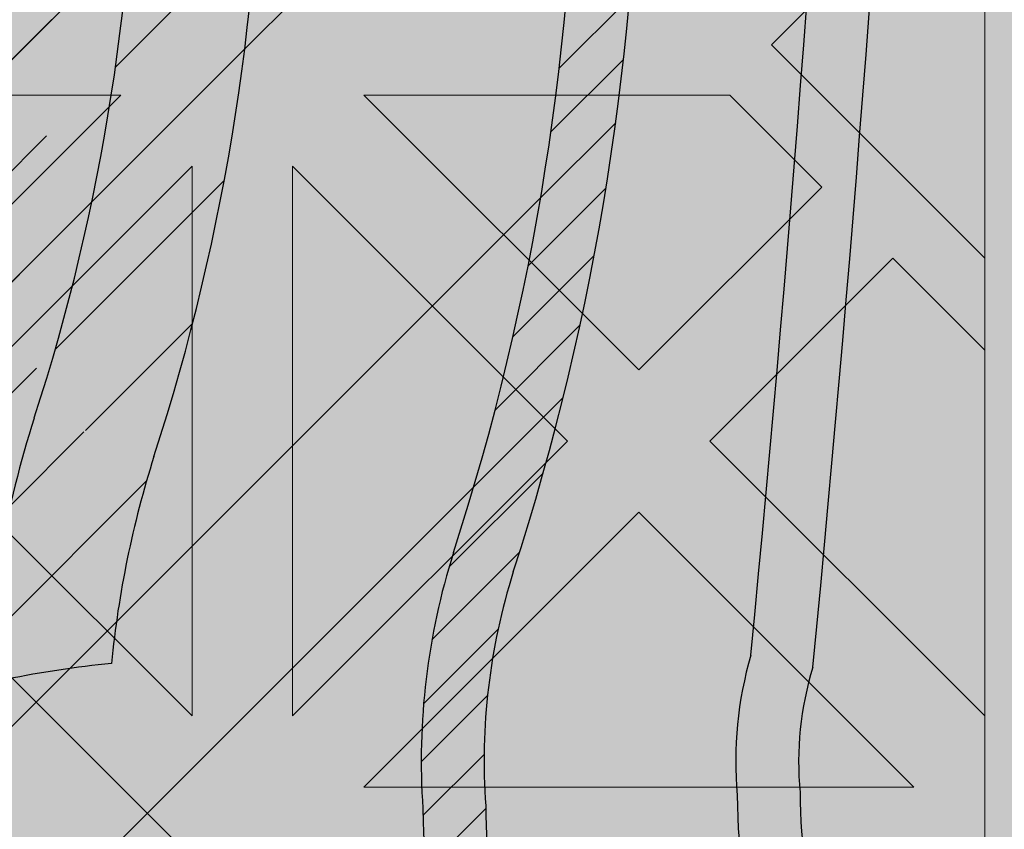
# Model space of a CAD drawing. Units: inches. Extents: x 844 to 2234, y 346 to 1084.
# Tile 54 of 93: x 1871.357 to 1873.853, y 694.275 to 696.327. Entities that reach past the tile are written whole.
import ezdxf

# ---------------------------------------------------------------- set-up
doc = ezdxf.new("R2010")
doc.units = ezdxf.units.IN
doc.header["$MEASUREMENT"] = 0
doc.layers.add('furniture', color=8, linetype='Continuous', lineweight=18)
doc.layers.add('RA-AP-01$0$INT', color=35, linetype='Continuous', lineweight=5)
doc.layers.add('RA-AP-01$0$FURN', color=3, linetype='Continuous')
doc.layers.add('RA-AP-01$0$WOOD', color=64, linetype='Continuous')

# ---------------------------------------------------------------- blocks, each defined once
blk = doc.blocks.new('A$C18D01794')
at = {"layer": 'RA-AP-01$0$INT'}
blk.add_hatch(color=256, dxfattribs=at).paths.add_polyline_path([(4.505206456958071, -6.306712009588038), (5.305206456958072, -6.306712009588038), (5.305206456958072, -7.106712009588038), (5.255206456951893, -7.10671200958804), (5.25520645694868, -6.356712009605972), (4.555206456959269, -6.356712009587461), (4.555206456956052, -7.106712009588038), (4.505206456958073, -7.106712009588038)])
h = blk.add_hatch(color=256, dxfattribs=at)
h.paths.add_polyline_path([(4.585917135068449, -6.356712009588271), (4.555206456959269, -6.35671200958746), (4.555206456959137, -6.387422687716308), (4.874495778835233, -6.706712009592356), (4.90520645695423, -6.676001331474049)])
h.paths.add_polyline_path([(5.255206456948813, -6.387422687716306), (5.255206456948682, -6.356712009605972), (5.224495778822613, -6.356712009605161), (4.905206456953498, -6.676001331474273), (4.935917135072151, -6.706712009592924)])
h.paths.add_polyline_path([(4.935917135072559, -6.706712009592068), (4.905206456953564, -6.737422687710376), (5.255206456951813, -7.087422687708613), (5.255206456951549, -7.026001331471008)])
h.paths.add_polyline_path([(4.555206456956399, -7.026001331471013), (4.555206456956134, -7.087422687708616), (4.905206456953821, -6.737422687710943), (4.874495778835166, -6.70671200959229)])
h = blk.add_hatch(color=256, dxfattribs=at)
h.paths.add_polyline_path([(4.585917135068448, -6.356712009588273), (4.614201406330596, -6.356712009589021), (4.668846067270487, -6.411356670531338), (4.723490728212344, -6.356712009591912), (4.771774999457151, -6.35671200959319), (4.826419660396886, -6.411356670535356), (4.862780050090322, -6.374996280843536), (4.844495778842715, -6.356712009595112), (4.862780050090411, -6.356712009595595), (4.905206456960182, -6.399138416468211), (4.947632863832445, -6.356712009597838), (4.965917135079675, -6.356712009598322), (4.947632863831759, -6.374996280845421), (4.983993253523576, -6.411356670538857), (5.038637914464627, -6.356712009600247), (5.08692218571208, -6.356712009601523), (5.141566846649976, -6.411356670541852), (5.196211507589851, -6.356712009604411), (5.224495778822615, -6.356712009605161), (4.905206456953975, -6.676001331473793)])
h.paths.add_polyline_path([(4.895206456956031, -6.637717060225675), (4.895206456958921, -6.528427738347902), (4.840561796018589, -6.583072399285802)], flags=16)
h.paths.add_polyline_path([(4.915206456955638, -6.637717060226121), (4.969851117895509, -6.583072399288678), (4.915206456957609, -6.528427738348344)], flags=16)
h.paths.add_polyline_path([(4.826419660395175, -6.568930263661755), (4.881064321335613, -6.514285602723745), (4.771774999456703, -6.514285602720857)], flags=16)
h.paths.add_polyline_path([(4.983993253519558, -6.568930263665262), (5.038637914460456, -6.514285602726792), (4.929348592581548, -6.514285602724816)], flags=16)
h.paths.add_polyline_path([(4.881064321336025, -6.494285602723742), (4.826419660397532, -6.439640941782821), (4.771774999457062, -6.494285602720859)], flags=16)
h.paths.add_polyline_path([(4.929348592582019, -6.494285602724817), (5.038637914460982, -6.494285602726792), (4.983993253522945, -6.439640941786327)], flags=16)
h.paths.add_polyline_path([(4.895206456960191, -6.480143467100443), (4.895206456962115, -6.407422687715913), (4.876922185715016, -6.389138416467584), (4.840561796021581, -6.425498806159401)], flags=16)
h.paths.add_polyline_path([(4.915206456958487, -6.480143467100889), (4.969851117899527, -6.425498806162279), (4.933490728206909, -6.389138416468043), (4.9152064569598, -6.40742268771434)], flags=16)
h.paths.add_polyline_path([(4.757632863832376, -6.480143467096812), (4.812277524772842, -6.425498806158772), (4.757632863834348, -6.370854145217844)], flags=16)
h.paths.add_polyline_path([(4.737632863832376, -6.480143467096286), (4.737632863834348, -6.370854145217375), (4.682988202893906, -6.425498806155385)], flags=16)
h.paths.add_polyline_path([(5.05278005008503, -6.480143467103376), (5.052780050087917, -6.370854145224413), (4.998135389146995, -6.425498806162908)], flags=16)
h.paths.add_polyline_path([(5.072780050085024, -6.480143467103744), (5.127424711025931, -6.42549880616527), (5.072780050087916, -6.370854145224832)], flags=16)
h.paths.add_polyline_path([(4.935917135072783, -6.706712009592292), (5.255206456948811, -6.387422687716309), (5.255206456948932, -6.415706958964177), (5.200561796010279, -6.470351619902839), (5.255206456949403, -6.524996280841948), (5.25520645694961, -6.5732805520894), (5.200561796009787, -6.627925213029239), (5.236922185702417, -6.664285602721864), (5.255206456949919, -6.646001331474357), (5.255206456949998, -6.664285602721898), (5.212780050078687, -6.706712009592262), (5.25520645695036, -6.749138416463932), (5.255206456950438, -6.767422687711313), (5.236922185702424, -6.749138416463297), (5.200561796009796, -6.785498806155928), (5.255206456950753, -6.840143467096874), (5.25520645695096, -6.888427738341682), (5.200561796010322, -6.943072399282328), (5.255206456951428, -6.997717060223427), (5.255206456951547, -7.026001331471006)])
h.paths.add_polyline_path([(5.042988202883395, -6.785498806155427), (5.097632863823085, -6.840143467095101), (5.097632863822622, -6.730854145216193)], flags=16)
h.paths.add_polyline_path([(5.028846067259663, -6.771356670531693), (5.083490728198774, -6.716712009592573), (4.974201406321001, -6.716712009593042)], flags=16)
h.paths.add_polyline_path([(5.117632863823087, -6.840143467095186), (5.172277524762331, -6.785498806155926), (5.11763286382262, -6.730854145216225)], flags=16)
h.paths.add_polyline_path([(5.08349072819877, -6.696712009593886), (5.028846067259652, -6.642067348654775), (4.974201406320998, -6.696712009593438)], flags=16)
h.paths.add_polyline_path([(5.131774999446817, -6.854285602718917), (5.186419660386065, -6.799640941779662), (5.241064321325782, -6.854285602719365)], flags=17)
h.paths.add_polyline_path([(5.131774999446228, -6.716712009592374), (5.186419660386065, -6.771356670532194), (5.222780050079488, -6.734996280838764), (5.204495778832781, -6.716712009592063)], flags=16)
h.paths.add_polyline_path([(5.097632863822613, -6.682569873970264), (5.097632863823061, -6.573280552091354), (5.042988202883383, -6.627925213031044)], flags=16)
h.paths.add_polyline_path([(5.131774999446899, -6.874285602718915), (5.241064321325809, -6.874285602719364), (5.186419660386591, -6.928930263658598)], flags=17)
h.paths.add_polyline_path([(5.131774999446226, -6.696712009594078), (5.204495778830767, -6.696712009594374), (5.22278005007868, -6.67842773834687), (5.186419660386049, -6.642067348654249)], flags=16)
h.paths.add_polyline_path([(5.11763286382262, -6.682569873970225), (5.17227752476232, -6.627925213030515), (5.117632863823064, -6.573280552091267)], flags=16)
h.paths.add_polyline_path([(5.186419660386069, -6.613783077405491), (5.241064321325754, -6.559138416465795), (5.131774999446791, -6.559138416466263)], flags=16)
h.paths.add_polyline_path([(5.131774999446872, -6.539138416466263), (5.24106432132578, -6.539138416465794), (5.186419660386554, -6.484493755526573)], flags=16)
h.paths.add_polyline_path([(5.255206456951811, -7.08742268770861), (5.255206456951895, -7.106712009588038), (4.555206456956052, -7.106712009588038), (4.555206456956136, -7.087422687708617), (4.905206456953973, -6.737422687710788)])
h.paths.add_polyline_path([(4.983993253513404, -6.8444937555241), (4.92934859257295, -6.899138416462108), (5.03863791445186, -6.899138416465014)], flags=16)
h.paths.add_polyline_path([(4.969851117889988, -6.83035161990006), (4.915206456952556, -6.775706958960171), (4.915206456949648, -6.884996280837944)], flags=16)
h.paths.add_polyline_path([(4.929348592572535, -6.919138416462105), (4.983993253511019, -6.973783077403037), (5.038637914451496, -6.919138416465012)], flags=16)
h.paths.add_polyline_path([(5.052780050074912, -6.93328055208906), (4.998135389134438, -6.987925213027088), (5.052780050072919, -7.042569873968025)], flags=16)
h.paths.add_polyline_path([(5.07278005007491, -6.933280552089588), (5.072780050072918, -7.042569873968497), (5.127424711013374, -6.987925213030498)], flags=16)
h.paths.add_polyline_path([(4.89520645695295, -6.775706958959721), (4.840561796013067, -6.830351619897157), (4.895206456950961, -6.884996280837494)], flags=16)
h.paths.add_polyline_path([(4.915206456948365, -6.933280552085403), (4.915206456946434, -7.006001331471951), (4.933490728192729, -7.024285602719066), (4.969851117886972, -6.987925213026453)], flags=16)
h.paths.add_polyline_path([(4.881064321327021, -6.899138416461022), (4.82641966038902, -6.84449375552057), (4.771774999448108, -6.899138416459029)], flags=16)
h.paths.add_polyline_path([(4.895206456950073, -6.933280552084951), (4.840561796009022, -6.987925213023558), (4.876922185700835, -7.024285602716997), (4.895206456948749, -7.006001331469487)], flags=16)
h.paths.add_polyline_path([(4.983993253510392, -7.0020673486505), (4.947632863816944, -7.038427738342319), (4.965917135064043, -7.05671200959023), (5.038637914448995, -7.056712009591555)], flags=16)
h.paths.add_polyline_path([(4.881064321326543, -6.91913841646102), (4.771774999447578, -6.919138416459031), (4.826419660385607, -6.973783077399508)], flags=16)
h.paths.add_polyline_path([(4.905206456946447, -7.014285602717636), (4.862780050074785, -7.056712009588352), (4.947632863816685, -7.056712009589775)], flags=16)
h.paths.add_polyline_path([(5.14156684663679, -7.002067348654549), (5.086922185696452, -7.056712009592438), (5.196211507574223, -7.056712009594425)], flags=16)
h.paths.add_polyline_path([(4.8264196603837, -7.002067348646972), (4.771774999442643, -7.056712009585575), (4.8444957788276, -7.056712009587508), (4.862780050075511, -7.038427738340416)], flags=16)
h.paths.add_polyline_path([(4.812277524760289, -6.98792521302292), (4.757632863822258, -6.933280552082447), (4.757632863819352, -7.042569873961408)], flags=16)
h.paths.add_polyline_path([(4.73763286382226, -6.933280552082079), (4.682988202881349, -6.987925213020536), (4.737632863819352, -7.04256987396099)], flags=16)
h.paths.add_polyline_path([(4.723490728195188, -7.056712009584289), (4.668846067257299, -7.002067348643949), (4.614201406317417, -7.056712009581383)], flags=16)
h.paths.add_polyline_path([(4.597632863829262, -6.706712009592262), (4.555206456957951, -6.664285602721896), (4.555206456958029, -6.646001331474357), (4.573490728205535, -6.664285602721864), (4.609851117898167, -6.627925213029238), (4.555206456958338, -6.573280552089402), (4.555206456958546, -6.524996280841952), (4.60985111789767, -6.470351619902839), (4.555206456959015, -6.415706958964177), (4.555206456959138, -6.387422687716309), (4.874495778835167, -6.70671200959229), (4.5552064569564, -7.026001331471015), (4.555206456956523, -6.997717060223433), (4.609851117897629, -6.94307239928233), (4.555206456956988, -6.888427738341681), (4.555206456957198, -6.840143467096881), (4.609851117898153, -6.78549880615593), (4.573490728205528, -6.749138416463297), (4.555206456957507, -6.76742268771132), (4.555206456957585, -6.749138416463933)])
h.paths.add_polyline_path([(4.712780050085332, -6.730854145216195), (4.712780050084863, -6.840143467095105), (4.767424711024555, -6.785498806155427)], flags=16)
h.paths.add_polyline_path([(4.726922185709173, -6.716712009592573), (4.781566846648288, -6.771356670531693), (4.836211507586949, -6.716712009593043)], flags=16)
h.paths.add_polyline_path([(4.692780050085327, -6.730854145216225), (4.638135389145619, -6.785498806155928), (4.692780050084865, -6.840143467095185)], flags=16)
h.paths.add_polyline_path([(4.726922185709182, -6.696712009593886), (4.836211507586949, -6.696712009593436), (4.7815668466483, -6.642067348654773)], flags=16)
h.paths.add_polyline_path([(4.678637914461726, -6.71671200959237), (4.605917135075169, -6.716712009592063), (4.587632863828464, -6.734996280838766), (4.623993253521887, -6.771356670532195)], flags=16)
h.paths.add_polyline_path([(4.712780050085336, -6.68256987397026), (4.767424711024568, -6.627925213031042), (4.71278005008489, -6.573280552091352)], flags=16)
h.paths.add_polyline_path([(4.678637914461726, -6.696712009594076), (4.623993253521899, -6.642067348654247), (4.587632863829271, -6.67842773834687), (4.605917135077185, -6.696712009594376)], flags=16)
h.paths.add_polyline_path([(4.692780050085336, -6.682569873970228), (4.692780050084889, -6.573280552091267), (4.638135389145632, -6.627925213030515)], flags=16)
h.paths.add_polyline_path([(4.623993253521885, -6.799640941779662), (4.678637914461131, -6.854285602718915), (4.56934859258217, -6.854285602719365)], flags=17)
h.paths.add_polyline_path([(4.623993253521901, -6.613783077405509), (4.678637914461158, -6.559138416466263), (4.569348592582195, -6.559138416465795)], flags=16)
h.paths.add_polyline_path([(4.678637914461051, -6.874285602718915), (4.623993253521361, -6.928930263658598), (4.569348592582143, -6.874285602719364)], flags=17)
h.paths.add_polyline_path([(4.678637914461076, -6.539138416466263), (4.623993253521399, -6.484493755526573), (4.569348592582167, -6.539138416465796)], flags=16)
h = blk.add_hatch(color=256, dxfattribs=at)
h.paths.add_polyline_path([(5.028846067259997, -6.642067348655121), (4.974201406321342, -6.696712009593783), (5.083490728199115, -6.69671200959423)])
h.paths.add_polyline_path([(4.974201406321344, -6.716712009593388), (5.028846067260004, -6.771356670532039), (5.083490728199117, -6.716712009592919)])
h.paths.add_polyline_path([(5.042988202883738, -6.785498806155768), (5.097632863823428, -6.840143467095449), (5.097632863822963, -6.73085414521654)])
h.paths.add_polyline_path([(5.117632863822961, -6.730854145216568), (5.117632863823428, -6.840143467095531), (5.172277524762674, -6.785498806156272)])
h.paths.add_polyline_path([(5.131774999446572, -6.716712009592718), (5.186419660386406, -6.77135667053254), (5.222780050079831, -6.734996280839116), (5.204495778833122, -6.716712009592409)])
h.paths.add_polyline_path([(5.236922185702764, -6.749138416463644), (5.200561796010139, -6.785498806156274), (5.255206456949971, -6.840143467096101), (5.255206456950271, -6.76742268771115)])
h.paths.add_polyline_path([(5.186419660386412, -6.799640941780006), (5.131774999447164, -6.854285602719262), (5.241064321326123, -6.854285602719711)])
h.paths.add_polyline_path([(5.131774999447238, -6.874285602719261), (5.186419660386934, -6.928930263658944), (5.241064321326153, -6.874285602719709)])
h.paths.add_polyline_path([(5.200561796010663, -6.943072399282675), (5.255206456949324, -6.997717060221329), (5.255206456949777, -6.888427738343558)])
h.paths.add_polyline_path([(5.21278005007903, -6.706712009592607), (5.255206456950223, -6.749138416463798), (5.255206456950696, -6.664285602721891)])
h.paths.add_polyline_path([(5.13177499944657, -6.696712009594424), (5.204495778831106, -6.696712009594723), (5.222780050079024, -6.678427738347219), (5.186419660386397, -6.642067348654592)])
h.paths.add_polyline_path([(5.117632863823405, -6.573280552091611), (5.117632863822955, -6.682569873970578), (5.172277524762665, -6.627925213030859)])
h.paths.add_polyline_path([(5.042988202883727, -6.627925213031387), (5.097632863822957, -6.682569873970603), (5.097632863823407, -6.573280552091697)])
h.paths.add_polyline_path([(5.131774999447135, -6.559138416466609), (5.186419660386394, -6.613783077405857), (5.241064321326097, -6.559138416466144)])
h.paths.add_polyline_path([(5.200561796010128, -6.627925213029584), (5.236922185702758, -6.664285602722211), (5.255206456950264, -6.646001331474705), (5.255206456949948, -6.573280552089752)])
h.paths.add_polyline_path([(5.186419660386895, -6.484493755526919), (5.131774999447213, -6.539138416466609), (5.241064321326127, -6.539138416466142)])
h.paths.add_polyline_path([(5.200561796010624, -6.470351619903183), (5.255206456949745, -6.524996280842298), (5.255206456949276, -6.415706958964523)])
for p, q in [((5.255206456951895, -7.106712009588038), (5.255206456948681, -6.356712009605972)), ((4.935917135072783, -6.706712009592292), (5.255206456948813, -6.387422687716307)), ((5.131774999446792, -6.559138416466263), (5.241064321325755, -6.559138416465795)), ((5.131774999446792, -6.559138416466263), (5.186419660386049, -6.613783077405509)), ((5.241064321325755, -6.559138416465795), (5.186419660386049, -6.613783077405509)), ((5.042988202883385, -6.627925213031041), (5.097632863823062, -6.573280552091352)), ((5.097632863823062, -6.573280552091352), (5.097632863822615, -6.682569873970262)), ((5.117632863823062, -6.573280552091267), (5.172277524762319, -6.627925213030515)), ((5.117632863823062, -6.573280552091267), (5.117632863822614, -6.68256987397023)), ((5.255206456949605, -6.573280552089405), (5.200561796009783, -6.627925213029239)), ((5.255206456949918, -6.646001331474357), (5.255206456949605, -6.573280552089405)), ((5.097632863822615, -6.682569873970262), (5.042988202883383, -6.627925213031042)), ((5.117632863822614, -6.68256987397023), (5.172277524762319, -6.627925213030515)), ((5.200561796009783, -6.627925213029238), (5.236922185702415, -6.664285602721863)), ((5.083490728198769, -6.696712009593882), (5.028846067259652, -6.642067348654775)), ((5.131774999446228, -6.696712009594078), (5.186419660386053, -6.642067348654247)), ((5.186419660386051, -6.642067348654247), (5.222780050078681, -6.67842773834687)), ((5.255206456949919, -6.646001331474357), (5.236922185702415, -6.664285602721864)), ((5.212780050078687, -6.706712009592262), (5.255206456950353, -6.664285602721543)), ((5.25520645694988, -6.74913841646345), (5.255206456950353, -6.664285602721543)), ((5.204495778833082, -6.69671200959206), (5.222780050078681, -6.67842773834687)), ((5.08349072819877, -6.696712009593886), (4.974201406320999, -6.696712009593436)), ((5.204495778831179, -6.696712009594376), (5.131774999446228, -6.696712009594078)), ((5.212780050078687, -6.706712009592262), (5.25520645694988, -6.74913841646345))]:
    blk.add_line(p, q, dxfattribs=at)
blk = doc.blocks.new('A$C32926AE1')
at = {"layer": 'RA-AP-01$0$FURN'}
h = blk.add_hatch(dxfattribs=at)
h.set_pattern_fill('ANSI31', color=256, scale=0.1, style=0)
h.set_pattern_definition([(45, (0, 0), (-0.0088388347648318, 0.0088388347648318), [])])
edge = h.paths.add_edge_path(flags=16)
edge.add_arc((4.904771284329206, 4.246793130718756), 0.2603971832811541, 75.22398030683196, 104.7760196931204)
edge.add_arc((4.904771284329206, 4.246793130718756), 0.2603971832811541, 75.223980306832, 104.77601969312039, ccw=False)
edge = h.paths.add_edge_path(flags=16)
edge.add_arc((4.904771284329206, 4.067062675376612), 0.2603971832811541, 255.2239803068796, 284.776019693168)
edge.add_arc((4.904771284329206, 4.067062675376612), 0.2603971832811541, 255.22398030687958, 284.77601969316805, ccw=False)
edge = h.paths.add_edge_path(flags=0)
edge.add_arc((4.904771284329206, 4.067062675376612), 0.2603971832811541, 255.2239803068796, 284.776019693168)
edge.add_arc((4.904771284329206, 4.067062675376612), 0.2603971832811541, 255.22398030687958, 284.77601969316805, ccw=False)
edge = h.paths.add_edge_path(flags=0)
edge.add_arc((4.904771284329206, 4.067062675376612), 0.2603971832811541, 255.2239803068796, 284.776019693168)
edge.add_arc((4.904771284329206, 4.067062675376612), 0.2603971832811541, 255.22398030687958, 284.77601969316805, ccw=False)
edge = h.paths.add_edge_path()
edge.add_arc((4.604388392048174, 4.588829985554312), 0.1599999999999918, 342.3781640246255, 354.4317409793762)
edge.add_arc((5.090145208887507, 4.43216705527679), 0.3503971832811637, 162.0091218307731, 180.3186872093483)
edge.add_arc((5.205154176610243, 4.588829985554953), 0.1599999999999917, 185.5682590208461, 197.6218359767349)
edge.add_arc((4.904771284329229, 4.246793130718735), 0.3503971832811761, 72.00912183053516, 107.9908781690354)
edge.add_arc((9.535952835716557, 4.28682295566602), 4.798342501046485, 178.2875002453811, 181.5576802719453)
edge.add_arc((4.719397359771122, 4.43216705527679), 0.3503971832811637, 359.6813127906516, 377.9908781692269)
edge.add_arc((9.535967292294904, 4.286822350292874), 4.778371420254705, 178.2965938931842, 181.5667745797229)
edge.add_arc((4.719397359771122, 4.43216705527679), 0.3303971832811637, 359.6813127906516, 377.9908781692269)
edge.add_arc((0.2735752763637294, 4.286822350292874), 4.7783714202547, 358.4332254202771, 361.7034061068158)
edge.add_arc((5.061434214606998, 4.732549947558029), 0.1600000000000254, 252.3781640250584, 264.4317409792362)
edge.add_arc((4.748108354051257, 4.732549947558012), 0.1600000000000541, 275.5682590208426, 287.6218359759532)
edge.add_arc((4.604388392048115, 4.588829985554317), 0.1800000000000505, 342.3567572500182, 349.3735009646207)
edge.add_arc((5.205154176610254, 4.588829985554976), 0.1800000000000069, 190.6264990356027, 197.6432427513933)
edge.add_arc((5.061434214607106, 4.732549947558013), 0.1800000000000424, 252.3567572496606, 259.3735009644582)
edge.add_arc((4.904771284329208, 4.246793130718737), 0.3303971832811676, 71.99844483668534, 108.0015551637021)
edge.add_arc((4.748108354051414, 4.732549947558045), 0.1800000000000547, 280.6264990355479, 287.6432427495938)
edge.add_arc((5.090145208887514, 4.432167055276789), 0.2803971832811691, 162.8706300666893, 180.816523289902)
edge.add_arc((4.719397359771136, 4.432167055276689), 0.2803971832811534, 359.183476710103, 377.1293699333214)
edge.add_arc((4.904771284329222, 4.246793130718737), 0.2803971832811769, 72.87063006672916, 107.1293699332334)
edge.add_arc((5.090145208887522, 4.432167055276788), 0.2603971832811776, 165.2239803068007, 180.9953123810312)
edge.add_arc((4.719397359771141, 4.432167055276699), 0.2603971832811458, 359.0046876189768, 374.7760196932087)
edge.add_arc((5.090145208887507, 4.43216705527679), 0.3303971832811637, 162.0091218307731, 180.3186872093483)
edge.add_arc((9.53595427642584, 4.285015535491528), 4.728345371032053, 178.265043920078, 181.5679956281801)
edge.add_arc((0.2735882922327999, 4.285015535491582), 4.728345371032045, 358.4320043718193, 361.7349560799204)
edge.add_arc((9.535953591267507, 4.284458026472751), 4.708343996644348, 178.2573054306777, 181.5704995759608)
edge.add_arc((0.273588977391114, 4.284458026472785), 4.708343996644358, 358.4295004240388, 361.7426945693213)
edge.add_arc((0.2735889773911131, 4.029397779622582), 4.708343996644359, 358.2573054306787, 361.5704995759613)
edge.add_arc((9.535953591267518, 4.029397779622618), 4.708343996644359, 178.4295004240391, 181.7426945693223)
edge.add_arc((0.2735882922327901, 4.028840270603786), 4.728345371032054, 358.2650439200796, 361.5679956281808)
edge.add_arc((9.53595427642584, 4.028840270603841), 4.728345371032054, 178.4320043718199, 181.7349560799219)
edge.add_arc((0.2735752763637302, 4.027033455802493), 4.778371420254699, 358.2965938931842, 361.5667745797229)
edge.add_arc((4.719397359771122, 3.881688750818578), 0.3303971832811637, 342.0091218307731, 360.3186872093484)
edge.add_arc((5.090145208887507, 3.881688750818578), 0.3303971832811637, 179.6813127906516, 197.9908781692269)
edge.add_arc((9.535967292294904, 4.027033455802493), 4.778371420254705, 178.433225420277, 181.7034061068158)
edge.add_arc((4.719397359771122, 3.881688750818578), 0.3503971832811637, 342.0091218307731, 360.3186872093484)
edge.add_arc((9.53595283571655, 4.027032850429349), 4.79834250104648, 178.4423197280546, 181.7124997546188)
edge.add_arc((4.719397359771141, 3.881688750818669), 0.2603971832811458, 345.2239803067913, 360.9953123810232)
edge.add_arc((5.090145208887522, 3.88168875081858), 0.2603971832811776, 179.0046876189687, 194.7760196931993)
edge.add_arc((4.904771284329222, 4.067062675376631), 0.2803971832811769, 252.8706300667665, 287.1293699332708)
edge.add_arc((4.719397359771136, 3.881688750818678), 0.2803971832811534, 342.8706300666787, 360.8165232898969)
edge.add_arc((5.090145208887514, 3.881688750818579), 0.2803971832811691, 179.183476710098, 197.1293699333106)
edge.add_arc((4.748108354051414, 3.581305858537323), 0.1800000000000547, 72.3567572504062, 79.37350096445199)
edge.add_arc((4.904771284329208, 4.067062675376631), 0.3303971832811676, 251.9984448362979, 288.0015551633146)
edge.add_arc((5.061434214607106, 3.581305858537355), 0.1800000000000424, 100.6264990355418, 107.6432427503394)
edge.add_arc((5.205154176610254, 3.725025820540392), 0.1800000000000069, 162.3567572486066, 169.3735009643972)
edge.add_arc((4.604388392048115, 3.725025820541051), 0.1800000000000505, 10.62649903537925, 17.64324274998182)
edge.add_arc((4.748108354051257, 3.581305858537356), 0.1600000000000541, 72.37816402404681, 84.43174097915735)
edge.add_arc((4.904771284329229, 4.067062675376632), 0.3503971832811761, 252.0091218309645, 287.9908781694648)
edge.add_arc((5.061434214606998, 3.581305858537339), 0.1600000000000254, 95.56825902076373, 107.6218359749416)
edge.add_arc((5.205154176610243, 3.725025820540414), 0.1599999999999917, 162.3781640232651, 174.4317409791539)
edge.add_arc((5.090145208887507, 3.881688750818578), 0.3503971832811637, 179.6813127906516, 197.9908781692269)
edge.add_arc((4.604388392048174, 3.725025820541056), 0.1599999999999918, 5.568259020623824, 17.62183597537444)
edge.add_arc((0.2735897329420762, 4.28682295566602), 4.798342501046482, 358.4423197280547, 361.7124997546188)
edge.add_arc((0.2735897329420691, 4.027032850429348), 4.798342501046489, 358.2875002453812, 361.5576802719453)
at = {"layer": 'RA-AP-01$0$WOOD'}
h = blk.add_hatch(color=256, dxfattribs=at)
h.dxf.hatch_style = 1
h.paths.add_polyline_path([(5.157430609644524, 4.573483066760929, -0.1009492694046607), (5.155401577623758, 4.593365984175333, -0.1842662638101597), (5.172249623284174, 4.638795604568598, 0.2056608120311276), (5.179560981299304, 4.661316324430096, 0.3614336704623542), (5.134352340494423, 4.706524965234944, 0.2056608120311297), (5.111831620632933, 4.699213607219793, -0.1842662638101113), (5.066402000239693, 4.682365561559342, -0.1055311479399994), (5.045656153913092, 4.68467289944697, 0.1567636581983829), (4.763886414745334, 4.684672899446966, -0.1055311479399895), (4.743140568418733, 4.68236556155934, -0.1842662638100833), (4.6977109480255, 4.69921360721979, 0.2056608120302612), (4.675190228164109, 4.706524965234949, 0.3614336704708441), (4.629981587358889, 4.66131632442871, 0.2056608120245944), (4.637292945374126, 4.638795604567974, -0.1842662638101024), (4.654140991034615, 4.59336598417475, -0.1009492694055169), (4.652111959013835, 4.573483066760181, 0.021410119221476), (4.629748025606143, 4.156712009541676, 0.0214101192214795), (4.652111959013809, 3.739940952323101, -0.1009492694059586), (4.654140991034615, 3.720058034908448, -0.1842662638100975), (4.637292945374126, 3.674628414515226, 0.2056608120245705), (4.629981587358889, 3.652107694654492, 0.3614336704708879), (4.675190228164113, 3.606899053848249, 0.2056608120302384), (4.697710948025501, 3.614210411863408, -0.1842662638100995), (4.743140568418738, 3.63105845752386, -0.1055311479402541), (4.763886414745388, 3.628751119636215, 0.1567636581983776), (5.045656153913137, 3.628751119636244, -0.1055311479397538), (5.066402000239692, 3.631058457523857, -0.1842662638101067), (5.111831620632931, 3.614210411863407, 0.2056608120310924), (5.134352340494417, 3.606899053848256, 0.3614336704624001), (5.179560981299307, 3.652107694653103, 0.2056608120311314), (5.172249623284175, 3.6746284145146, -0.1842662638101402), (5.155401577623758, 3.72005803490786, -0.1009492694051366), (5.15743060964455, 3.739940952322354, 0.0214101192215073), (5.179794543052287, 4.156712009541468, 0.0214101192215252)])
h.paths.add_polyline_path([(4.639748609479751, 4.156712009541513, 0.0213537860821624), (4.661970494867118, 3.741887061152232, -0.094075836301374), (4.664143710413708, 3.7196126951003, -0.1824818158568985), (4.644813765429836, 3.668037719127816, 0.2056608120245319), (4.639939526753007, 3.653023905887301, 0.3614336704710246), (4.676106439397173, 3.616856993242342, 0.2056608120302234), (4.691120252638095, 3.621731231919122, -0.1824818158602558), (4.742695228611606, 3.641061176902986, -0.1029891339458722), (4.766991894714349, 3.638256818950944, 0.156709409989566), (5.042550673941472, 3.638256818950105, -0.102989133958497), (5.066847340047078, 3.641061176902949, -0.1824818158594995), (5.118422316020358, 3.621731231919103, 0.2056608120311416), (5.133436129261316, 3.616856993242346, 0.3614336704621468), (5.169603041905217, 3.653023905886178, 0.2056608120310986), (5.164728803228477, 3.668037719127177, -0.1824818158565612), (5.145398858244737, 3.719612695099578, -0.0940758363009313), (5.147572073791232, 3.741887061151398, 0.0213537860822023), (5.169793959178681, 4.156712009541451, 0.0213537860822226), (5.147572073791203, 4.571536957931898, -0.0940758363005034), (5.145398858244737, 4.59381132398362, -0.1824818158565587), (5.164728803228476, 4.645386299956021, 0.2056608120311045), (5.169603041905216, 4.66040011319702, 0.3614336704621845), (5.133436129261313, 4.696567025840856, 0.2056608120310773), (5.118422316020359, 4.691692787164098, -0.182481815859508), (5.066847340047078, 4.67236284218025, -0.1029891339584606), (5.04255067394148, 4.675167200133092, 0.156709409989566), (4.766991894714357, 4.675167200132257, -0.1029891339458842), (4.742695228611611, 4.672362842180213, -0.1824818158602725), (4.691120252638095, 4.691692787164077, 0.2056608120302152), (4.676106439397174, 4.696567025840858, 0.3614336704710363), (4.639939526753005, 4.660400113195899, 0.2056608120245495), (4.644813765429837, 4.645386299955384, -0.1824818158568934), (4.664143710413708, 4.593811323982902, -0.0940758363009187), (4.661970494867149, 4.571536957931074, 0.021353786082177)], flags=16)
h.paths.add_polyline_path([(5.129794543052235, 4.432167055276933, -0.0141661062790638), (5.130152669293814, 4.156927903047693, -0.0141661062790647), (5.129794543052234, 3.881688750818433, -0.0785247771143638), (5.10979738006795, 3.755143611847103, 0.0945969212073497), (5.105408519571111, 3.717898134952927, 0.1043170707844957), (5.116074640131521, 3.670385395016088, 0.1043170707864965), (5.068561900193738, 3.681051515576561, 0.09459692119553), (5.031316423304057, 3.676662655080835, -0.1580239521427272), (4.778226145355827, 3.676662655080367, 0.0945969211986668), (4.740980668464973, 3.681051515576592, 0.1043170707882822), (4.693467928526415, 3.670385395015844, 0.1043170707867916), (4.704134049087309, 3.717898134953662, 0.0945969211972894), (4.69974518859162, 3.755143611844042, -0.0785247771163196), (4.679748025606343, 3.881688750818406, -0.0141661062790663), (4.679389899364763, 4.156927903047693, -0.0141661062790672), (4.679748025606343, 4.432167055276998, -0.0785247771163064), (4.699745188591625, 4.55871219425134, 0.094596921197333), (4.704134049087308, 4.595957671141738, 0.1043170707867205), (4.693467928526416, 4.643470411079523, 0.1043170707882628), (4.740980668464965, 4.632804290518776, 0.0945969211988114), (4.778226145355874, 4.637193151015016, -0.158023952142669), (5.031316423304015, 4.637193151014546, 0.0945969211956361), (5.068561900193736, 4.632804290518806, 0.1043170707864979), (5.11607464013152, 4.643470411079278, 0.1043170707844617), (5.105408519571112, 4.595957671142455, 0.0945969212074597), (5.109797380067959, 4.558712194248236, -0.0785247771143467)], flags=0)
h.paths.add_polyline_path([(5.119794532311105, 4.432259799204851, -0.0142000800617244), (5.120156169157484, 4.156927903047701, -0.0142000800617277), (5.119794532311105, 3.881596006890482, -0.0784894509520253), (5.100273383573699, 3.758192358677797, 0.0940138827242913), (5.095413455884425, 3.717477693979438, 0.0606271852308753), (5.099615656341024, 3.686844378806616, 0.0606271852322524), (5.068982341167493, 3.691046579263239, 0.0940138827010453), (5.028267676478798, 3.686186651576848, -0.1580706864508061), (4.781274892180912, 3.686186651576435, 0.0940138827026903), (4.740560227491556, 3.691046579263279, 0.0606271852339895), (4.709926912317155, 3.686844378806508, 0.0606271852329405), (4.714129112773991, 3.717477693980356, 0.094013882701304), (4.709269185087677, 3.758192358669163, -0.0784894509577193), (4.689748036347473, 3.881596006890469, -0.014200080061729), (4.689386399501094, 4.156927903047709, -0.0142000800617217), (4.689748036347473, 4.432259799204808, -0.078489450957724), (4.709269185087651, 4.555663447426125, 0.0940138827014585), (4.714129112773992, 4.596378112114996, 0.0606271852329731), (4.709926912317154, 4.62701142728886, 0.0606271852340196), (4.74056022749157, 4.622809226832087, 0.0940138827024997), (4.781274892180847, 4.627669154518912, -0.1580706864508359), (5.028267676478777, 4.627669154518526, 0.0940138827010946), (5.068982341167492, 4.622809226832129, 0.060627185232254), (5.099615656341024, 4.627011427288751, 0.0606271852308727), (5.095413455884425, 4.59637811211593, 0.0940138827241088), (5.100273383573675, 4.555663447417647, -0.0784894509520978)], flags=0)
h.paths.add_polyline_path([(5.06978912287499, 4.430218106756144, -0.014241683694547), (5.070173729147532, 4.156927903047672, -0.0142416836945458), (5.06978912287499, 3.883637699339223, -0.0800609523125196), (5.052662118612511, 3.773463122773442, 0.0526421978001116), (5.04590916754064, 3.740550867606997, 0.0526421977992423), (5.012996912374707, 3.73379791653534, -0.1583028414718258), (4.796545656286308, 3.73379791653451, 0.0526421978034211), (4.763633401117837, 3.740550867607021, 0.0526421978018622), (4.756880450045755, 3.773463122774558, -0.0800609523117106), (4.739753445783639, 3.883637699339268, -0.0142416836945435), (4.739368839511098, 4.156927903047671, -0.0142416836945477), (4.739753445783639, 4.430218106756155, -0.0800609523116345), (4.75688045004574, 4.540392683320762, 0.052642197801941), (4.763633401117837, 4.573304938488346, 0.0526421978035071), (4.796545656286361, 4.580057889560873, -0.1583028414717561), (5.012996912374669, 4.580057889560039, 0.0526421977993048), (5.04590916754064, 4.57330493848837, 0.0526421978002057), (5.052662118612529, 4.540392683321868, -0.080060952312477)], flags=0)
h.paths.add_polyline_path([(5.049789715110557, 4.43038092723357, -0.0143097550741839), (5.05018085590259, 4.156927903047715, -0.0143097550741854), (5.049789715110558, 3.883474878861827, -0.0800685599149176), (5.03362098255317, 3.779581877367999, 0.0306258898956367), (5.028241146483733, 3.758218888663947, 0.0306258898977031), (5.006878157778253, 3.75283905259408, -0.1583983521624096), (4.802664410878162, 3.752839052594731, 0.0306258898946014), (4.781301422174808, 3.758218888663924, 0.0306258898967912), (4.775921586105202, 3.779581877368794, -0.080068559914251), (4.759752853548071, 3.883474878861786, -0.0143097550741854), (4.759361712756037, 4.156927903047671, -0.0143097550741854), (4.759752853548071, 4.430380927233557, -0.0800685599142479), (4.775921586105193, 4.534273928726546, 0.0306258898968306), (4.781301422174808, 4.555636917431444, 0.0306258898945754), (4.802664410878143, 4.561016753500631, -0.1583983521624168), (5.006878157778244, 4.561016753501291, 0.0306258898977177), (5.028241146483733, 4.555636917431421, 0.0306258898958182), (5.03362098255321, 4.534273928727244, -0.080068559914796)], flags=0)
h.paths.add_polyline_path([(4.999766070382627, 4.428171244713864, -0.0143443147609634), (5.000198441819402, 4.156927903047689, -0.0143443147609612), (4.999766070382627, 3.885684561381556, -0.0784641635803329), (4.987356730658798, 3.799103304488872, -0.1506053783831347), (4.822185837999821, 3.79910330448882, -0.0784641635803318), (4.809776498276007, 3.885684561381509, -0.014344314760963), (4.809344126839227, 4.156927903047677, -0.0143443147609645), (4.809776498276007, 4.428171244713873, -0.0784641635803192), (4.822185837999822, 4.514752501606549, -0.1506053783831338), (4.987356730658798, 4.514752501606494, -0.078464163580285)], flags=0)
h.paths.add_polyline_path([(4.979755254238824, 4.42764379880488, -0.0143772539198268), (4.980205517789977, 4.156927903047693, -0.0143772539198275), (4.979755254238824, 3.886212007290489, -0.0689242507424422), (4.971183264704897, 3.815276770442801, -0.1296645318904179), (4.838359303953726, 3.815276770442746, -0.0689242507424186), (4.829787314419809, 3.886212007290419, -0.0143772539198292), (4.829337050868653, 4.156927903047653, -0.0143772539198325), (4.829787314419809, 4.427643798804946, -0.0689242507424211), (4.838359303953725, 4.498579035652621, -0.1296645318904187), (4.971183264704897, 4.498579035652565, -0.0689242507424401)], flags=0)
h = blk.add_hatch(color=256, dxfattribs=at)
h.dxf.hatch_style = 1
h.paths.add_polyline_path([(5.145398858244737, 4.59381132398362, -0.1824818158565616), (5.164728803228476, 4.645386299956021, 0.2056608120311045), (5.169603041905216, 4.66040011319702, 0.3614336704621845), (5.133436129261313, 4.696567025840856, 0.2056608120310773), (5.118422316020359, 4.691692787164098, -0.182481815859508), (5.066847340047078, 4.67236284218025, -0.1029891339584606), (5.04255067394148, 4.675167200133092, 0.156709409989566), (4.766991894714357, 4.675167200132257, -0.1029891339458842), (4.742695228611611, 4.672362842180213, -0.1824818158602725), (4.691120252638095, 4.691692787164077, 0.2056608120302152), (4.676106439397174, 4.696567025840858, 0.3614336704710363), (4.639939526753005, 4.660400113195899, 0.2056608120245495), (4.644813765429837, 4.645386299955384, -0.1824818158568934), (4.664143710413708, 4.593811323982902, -0.0940758363009187), (4.661970494867149, 4.571536957931074, 0.0213537860821772), (4.639748609479751, 4.156712009541507, 0.0213537860821625), (4.661970494867119, 3.741887061152226, -0.0940758363013071), (4.664143710413708, 3.719612695100309, -0.1824818158569294), (4.644813765429836, 3.668037719127816, 0.2056608120245319), (4.639939526753007, 3.653023905887301, 0.3614336704710246), (4.676106439397173, 3.616856993242342, 0.2056608120302234), (4.691120252638095, 3.621731231919122, -0.1824818158602558), (4.742695228611606, 3.641061176902986, -0.1029891339458722), (4.766991894714349, 3.638256818950944, 0.156709409989566), (5.042550673941472, 3.638256818950105, -0.102989133958497), (5.066847340047078, 3.641061176902949, -0.1824818158594995), (5.118422316020358, 3.621731231919103, 0.2056608120311416), (5.133436129261316, 3.616856993242346, 0.3614336704621468), (5.169603041905217, 3.653023905886178, 0.2056608120310986), (5.164728803228477, 3.668037719127177, -0.1824818158565612), (5.145398858244737, 3.719612695099578, -0.0940758363009313), (5.147572073791232, 3.741887061151398, 0.0213537860822023), (5.169793959178681, 4.156712009541451, 0.0213537860822226), (5.147572073791203, 4.571536957931898, -0.0940758363004996)])
h.paths.add_polyline_path([(5.109797380067958, 4.55871219424824, -0.0785247771143472), (5.129794543052234, 4.432167055276936, -0.0141661062790644), (5.130152669293814, 4.156927903047685, -0.014166106279066), (5.129794543052234, 3.881688750818401, -0.0785247771143517), (5.109797380067946, 3.755143611847092, 0.0945969212073132), (5.105408519571111, 3.717898134952929, 0.1043170707844995), (5.116074640131521, 3.670385395016088, 0.1043170707864965), (5.068561900193738, 3.681051515576561, 0.09459692119553), (5.031316423304057, 3.676662655080835, -0.1580239521427272), (4.778226145355827, 3.676662655080367, 0.0945969211986668), (4.740980668464973, 3.681051515576592, 0.1043170707882822), (4.693467928526415, 3.670385395015844, 0.1043170707867916), (4.704134049087309, 3.717898134953662, 0.0945969211972894), (4.69974518859162, 3.755143611844042, -0.0785247771163196), (4.679748025606343, 3.881688750818406, -0.0141661062790663), (4.679389899364763, 4.156927903047693, -0.0141661062790672), (4.679748025606343, 4.432167055276998, -0.0785247771163064), (4.699745188591625, 4.55871219425134, 0.094596921197333), (4.704134049087308, 4.595957671141738, 0.1043170707867205), (4.693467928526416, 4.643470411079523, 0.1043170707882628), (4.740980668464965, 4.632804290518776, 0.0945969211988114), (4.778226145355874, 4.637193151015016, -0.158023952142669), (5.031316423304015, 4.637193151014546, 0.0945969211956361), (5.068561900193736, 4.632804290518806, 0.1043170707864979), (5.11607464013152, 4.643470411079278, 0.1043170707844617), (5.105408519571112, 4.595957671142455, 0.0945969212074504)], flags=16)
h.paths.add_polyline_path([(5.100273383573655, 4.55566344741771, -0.0784894509521388), (5.119794532311105, 4.432259799204852, -0.0142000800617252), (5.120156169157484, 4.156927903047686, -0.014200080061726), (5.119794532311105, 3.881596006890502, -0.0784894509520446), (5.100273383573696, 3.758192358677786, 0.0940138827242721), (5.095413455884425, 3.717477693979436, 0.0606271852308692), (5.099615656341024, 3.686844378806616, 0.0606271852322522), (5.068982341167493, 3.691046579263239, 0.0940138827010453), (5.028267676478798, 3.686186651576848, -0.1580706864508061), (4.781274892180912, 3.686186651576435, 0.0940138827026903), (4.740560227491556, 3.691046579263279, 0.0606271852339895), (4.709926912317155, 3.686844378806508, 0.0606271852329405), (4.714129112773991, 3.717477693980356, 0.094013882701304), (4.709269185087677, 3.758192358669163, -0.0784894509577193), (4.689748036347473, 3.881596006890469, -0.014200080061729), (4.689386399501094, 4.156927903047709, -0.0142000800617217), (4.689748036347473, 4.432259799204808, -0.078489450957724), (4.709269185087651, 4.555663447426125, 0.0940138827014585), (4.714129112773992, 4.596378112114996, 0.0606271852329731), (4.709926912317154, 4.62701142728886, 0.0606271852340196), (4.74056022749157, 4.622809226832087, 0.0940138827024997), (4.781274892180847, 4.627669154518912, -0.1580706864508359), (5.028267676478777, 4.627669154518526, 0.0940138827010946), (5.068982341167492, 4.622809226832129, 0.060627185232254), (5.099615656341024, 4.627011427288751, 0.0606271852308727), (5.095413455884425, 4.59637811211593, 0.094013882723957)], flags=0)
h.paths.add_polyline_path([(5.04590916754064, 4.57330493848837, 0.0526421978002057), (5.052662118612529, 4.540392683321868, -0.0800609523124783), (5.06978912287499, 4.430218106756142, -0.0142416836945469), (5.070173729147532, 4.156927903047672, -0.0142416836945458), (5.06978912287499, 3.883637699339223, -0.0800609523125196), (5.052662118612511, 3.773463122773442, 0.0526421978001116), (5.04590916754064, 3.740550867606997, 0.0526421977992423), (5.012996912374707, 3.73379791653534, -0.1583028414718258), (4.796545656286308, 3.73379791653451, 0.0526421978034211), (4.763633401117837, 3.740550867607021, 0.0526421978018622), (4.756880450045755, 3.773463122774558, -0.0800609523117106), (4.739753445783639, 3.883637699339268, -0.0142416836945435), (4.739368839511098, 4.156927903047671, -0.0142416836945477), (4.739753445783639, 4.430218106756155, -0.0800609523116345), (4.75688045004574, 4.540392683320762, 0.052642197801941), (4.763633401117837, 4.573304938488346, 0.0526421978035071), (4.796545656286361, 4.580057889560873, -0.1583028414717561), (5.012996912374669, 4.580057889560039, 0.0526421977993048)], flags=0)
h.paths.add_polyline_path([(5.028241146483733, 4.555636917431422, 0.0306258898956949), (5.033620982553182, 4.534273928727329, -0.0800685599148649), (5.049789715110557, 4.430380927233569, -0.0143097550741839), (5.05018085590259, 4.156927903047715, -0.0143097550741854), (5.049789715110558, 3.883474878861827, -0.0800685599149176), (5.03362098255317, 3.779581877367999, 0.0306258898956367), (5.028241146483733, 3.758218888663947, 0.0306258898977031), (5.006878157778253, 3.75283905259408, -0.1583983521624096), (4.802664410878162, 3.752839052594731, 0.0306258898946014), (4.781301422174808, 3.758218888663924, 0.0306258898967912), (4.775921586105202, 3.779581877368794, -0.080068559914251), (4.759752853548071, 3.883474878861786, -0.0143097550741854), (4.759361712756037, 4.156927903047671, -0.0143097550741854), (4.759752853548071, 4.430380927233557, -0.0800685599142479), (4.775921586105193, 4.534273928726546, 0.0306258898968306), (4.781301422174808, 4.555636917431444, 0.0306258898945754), (4.802664410878143, 4.561016753500631, -0.1583983521624168), (5.006878157778244, 4.561016753501291, 0.0306258898977174)], flags=0)
h.paths.add_polyline_path([(4.987356730658798, 4.514752501606494, -0.0784641635803018), (4.999766070382627, 4.428171244713845, -0.0143443147609637), (5.000198441819402, 4.156927903047665, -0.0143443147609622), (4.999766070382628, 3.885684561381514, -0.0784641635802952), (4.987356730658797, 3.799103304488872, -0.1506053783831338), (4.822185837999821, 3.799103304488819, -0.0784641635803342), (4.809776498276007, 3.885684561381512, -0.0143443147609628), (4.809344126839227, 4.156927903047676, -0.0143443147609646), (4.809776498276007, 4.428171244713873, -0.0784641635803192), (4.822185837999822, 4.514752501606549, -0.1506053783831338)], flags=0)
h.paths.add_polyline_path([(4.971183264704897, 4.498579035652566, -0.0689242507424384), (4.979755254238824, 4.427643798804883, -0.0143772539198276), (4.980205517789977, 4.15692790304768, -0.0143772539198258), (4.979755254238823, 3.88621200729051, -0.0689242507424628), (4.971183264704897, 3.815276770442801, -0.129664531890417), (4.838359303953726, 3.815276770442746, -0.0689242507424186), (4.829787314419809, 3.886212007290419, -0.0143772539198292), (4.829337050868653, 4.156927903047653, -0.0143772539198325), (4.829787314419809, 4.427643798804946, -0.0689242507424211), (4.838359303953725, 4.498579035652621, -0.1296645318904187)], flags=0)
h = blk.add_hatch(dxfattribs=at)
h.set_pattern_fill('ANSI31', color=256, scale=0.05, style=0)
h.set_pattern_definition([(45, (0, 0), (-0.0044194173824159, 0.0044194173824159), [])])
h.paths.add_polyline_path([(5.130152669293814, 4.156927903047704, 0.0141661062790657), (5.129794543052234, 4.432167055276982, 0.0777827904001433), (5.110168979996553, 4.557559993161921, -0.0976515123401879), (5.105408519571111, 4.595957671142454, -0.1043170707844687), (5.116074640131522, 4.64347041107928), (5.099615656341024, 4.627011427288751, 0.0606271852308727), (5.095413455884425, 4.59637811211593, 0.0940138827241088), (5.100273383573675, 4.555663447417647, -0.0784894509520972), (5.119794532311105, 4.432259799204852, -0.0142000800617252), (5.120156169157484, 4.156927903047686, -0.014200080061726), (5.119794532311105, 3.881596006890502, -0.0784894509520446), (5.100273383573696, 3.758192358677786, 0.0940138827242721), (5.095413455884425, 3.717477693979436, 0.0606271852308692), (5.099615656341024, 3.686844378806616), (5.116074640131519, 3.67038539501609, -0.1043170707844594), (5.105408519571112, 3.717898134952912, -0.0976515123401594), (5.11016897999655, 3.756295812933435, 0.0777827904001654), (5.129794543052234, 3.881688750818409, 0.0141661062790665)])
h.paths.add_polyline_path([(5.030164222210597, 3.676291055149937, -0.0976515123472002), (5.068561900193739, 3.681051515576561, -0.1043170707864927), (5.116074640131521, 3.670385395016088), (5.099615656341024, 3.686844378806616, 0.0606271852322522), (5.068982341167493, 3.691046579263239, 0.0940138827010453), (5.028267676478798, 3.686186651576848, -0.1580706864508061), (4.781274892180912, 3.686186651576435, 0.0940138827026903), (4.740560227491556, 3.691046579263279, 0.0606271852339913), (4.709926912317154, 3.686844378806508), (4.693467928526416, 3.670385395015845, -0.1043170707882796), (4.740980668464973, 3.681051515576592, -0.0976515123427246), (4.779378346446416, 3.676291055150394, 0.156512506893803)])
h.paths.add_polyline_path([(4.689748036347473, 3.881596006890472, -0.014200080061729), (4.689386399501094, 4.156927903047712, -0.0142000800617195), (4.689748036347473, 4.432259799204768, -0.078489450957742), (4.709269185087648, 4.555663447426114, 0.0940138827014821), (4.714129112773992, 4.596378112114995, 0.0606271852329748), (4.709926912317154, 4.62701142728886), (4.693467928526414, 4.643470411079524, -0.1043170707867939), (4.704134049087309, 4.595957671141706, -0.09765151234893), (4.699373588660725, 4.557559993157876, 0.0777827903975372), (4.679748025606343, 4.432167055276987, 0.0141661062790675), (4.679389899364763, 4.156927903047675, 0.0141661062790641), (4.679748025606343, 3.88168875081843, 0.0777827903975637), (4.699373588660724, 3.756295812937497, -0.0976515123490278), (4.704134049087308, 3.717898134953629, -0.1043170707867196), (4.693467928526416, 3.670385395015845), (4.709926912317155, 3.686844378806508, 0.0606271852329413), (4.714129112773991, 3.717477693980357, 0.0940138827013084), (4.709269185087676, 3.758192358669166, -0.0784894509577192)])
h.paths.add_polyline_path([(4.779378346446434, 4.63756475094498, -0.0976515123427943), (4.740980668464964, 4.632804290518776, -0.1043170707882609), (4.693467928526416, 4.643470411079523), (4.709926912317154, 4.62701142728886, 0.0606271852340196), (4.74056022749157, 4.622809226832087, 0.0940138827024997), (4.781274892180847, 4.627669154518912, -0.1580706864508359), (5.028267676478777, 4.627669154518526, 0.0940138827010946), (5.068982341167492, 4.622809226832129, 0.060627185232254), (5.099615656341024, 4.627011427288751), (5.116074640131521, 4.643470411079279, -0.1043170707865022), (5.068561900193735, 4.632804290518806, -0.0976515123475899), (5.030164222210446, 4.637564750945479, 0.1565125068936924)])
h = blk.add_hatch(dxfattribs=at)
h.set_pattern_fill('ANSI32', color=256, scale=0.2, style=0)
h.set_pattern_definition([(45, (0, 0), (-0.0530330085889911, 0.0530330085889911), []), (45, (0.035355339, 0), (-0.0530330085889911, 0.0530330085889911), [])])
h.paths.add_polyline_path([(5.119794532311105, 4.432259799204823, 0.0777015974868765), (5.10065834347252, 4.554469821747928, -0.0968902511992216), (5.095413455884425, 4.596378112115931, -0.060627185230871), (5.099615656341024, 4.627011427288751, -0.060627185232254), (5.068982341167492, 4.622809226832129, -0.0968902512198245), (5.027074050790956, 4.628054114423209, 0.1564657949319105), (4.782468517866163, 4.628054114422785, -0.0968902512152247), (4.740560227491555, 4.622809226832088, -0.0606271852339878), (4.709926912317155, 4.627011427288859, -0.0606271852329413), (4.714129112773991, 4.596378112115011, -0.0968902512205338), (4.708884225182929, 4.554469821738175, 0.0777015974804443), (4.689748036347473, 4.43225979920482, 0.0142000800617215), (4.689386399501094, 4.156927903047726, 0.0142000800617273), (4.689748036347473, 3.88159600689052, 0.077701597480541), (4.708884225182985, 3.759385984357019, -0.096890251220082), (4.714129112773992, 3.717477693980371, -0.0606271852329731), (4.709926912317154, 3.686844378806507, -0.060627185233988), (4.740560227491554, 3.691046579263279, -0.0968902512152569), (4.782468517866175, 3.685801691672578, 0.1564657949319236), (5.027074050790988, 3.685801691672169, -0.0968902512197451), (5.068982341167491, 3.691046579263239, -0.0606271852322557), (5.099615656341024, 3.686844378806616, -0.0606271852308727), (5.095413455884425, 3.717477693979438, -0.0968902511991229), (5.100658343472507, 3.7593859843474, 0.0777015974868745), (5.119794532311105, 3.8815960068905, 0.014200080061726), (5.120156169157484, 4.156927903047685, 0.0142000800617238)])
h.paths.add_polyline_path([(5.070173729147531, 4.156927903047684, -0.0142416836945481), (5.06978912287499, 3.883637699339191, -0.0800609523125107), (5.052662118612505, 3.773463122773424, 0.0526421978000811), (5.04590916754064, 3.740550867606997, 0.0526421977993214), (5.012996912374658, 3.733797916535325, -0.1583028414717916), (4.796545656286304, 3.733797916534512, 0.0526421978034138), (4.763633401117837, 3.740550867607021, 0.0526421978018622), (4.756880450045755, 3.773463122774558, -0.0800609523117106), (4.739753445783639, 3.883637699339268, -0.0142416836945435), (4.739368839511098, 4.156927903047671, -0.0142416836945477), (4.739753445783639, 4.430218106756155, -0.0800609523116345), (4.75688045004574, 4.540392683320762, 0.052642197801941), (4.763633401117837, 4.573304938488346, 0.0526421978035071), (4.796545656286361, 4.580057889560873, -0.1583028414717561), (5.012996912374669, 4.580057889560039, 0.0526421977993048), (5.04590916754064, 4.57330493848837, 0.0526421978002057), (5.052662118612529, 4.540392683321868, -0.0800609523124783), (5.06978912287499, 4.430218106756142, -0.0142416836945463)], flags=16)
h.paths.add_polyline_path([(5.050180855902591, 4.156927903047686, -0.0143097550741856), (5.049789715110558, 3.883474878861795, -0.0800685599148126), (5.033620982553202, 3.7795818773681, 0.0306258898957837), (5.028241146483733, 3.758218888663947, 0.0306258898977031), (5.006878157778253, 3.75283905259408, -0.1583983521624096), (4.802664410878162, 3.752839052594731, 0.0306258898946014), (4.781301422174808, 3.758218888663924, 0.0306258898967912), (4.775921586105202, 3.779581877368794, -0.080068559914251), (4.759752853548071, 3.883474878861786, -0.0143097550741854), (4.759361712756037, 4.156927903047671, -0.0143097550741854), (4.759752853548071, 4.430380927233557, -0.0800685599142479), (4.775921586105193, 4.534273928726546, 0.0306258898968306), (4.781301422174808, 4.555636917431444, 0.0306258898945754), (4.802664410878143, 4.561016753500631, -0.1583983521624168), (5.006878157778244, 4.561016753501291, 0.0306258898977177), (5.028241146483733, 4.555636917431421, 0.0306258898958182), (5.03362098255321, 4.534273928727244, -0.0800685599147973), (5.049789715110557, 4.430380927233568, -0.0143097550741854)], flags=0)
h.paths.add_polyline_path([(5.000198441819402, 4.15692790304769, -0.0143443147609622), (4.999766070382627, 3.885684561381539, -0.0784641635803169), (4.987356730658798, 3.799103304488873, -0.1506053783831347), (4.822185837999821, 3.79910330448882, -0.0784641635803318), (4.809776498276007, 3.885684561381509, -0.014344314760963), (4.809344126839227, 4.156927903047677, -0.0143443147609645), (4.809776498276007, 4.428171244713873, -0.0784641635803192), (4.822185837999822, 4.514752501606549, -0.1506053783831338), (4.987356730658798, 4.514752501606494, -0.0784641635803018), (4.999766070382627, 4.428171244713845, -0.0143443147609624)], flags=0)
h.paths.add_polyline_path([(4.980205517789976, 4.156927903047707, -0.0143772539198295), (4.979755254238824, 3.886212007290466, -0.06892425074242), (4.971183264704897, 3.815276770442801, -0.129664531890417), (4.838359303953726, 3.815276770442746, -0.0689242507424186), (4.829787314419809, 3.886212007290419, -0.0143772539198292), (4.829337050868653, 4.156927903047653, -0.0143772539198325), (4.829787314419809, 4.427643798804946, -0.0689242507424211), (4.838359303953725, 4.498579035652621, -0.1296645318904187), (4.971183264704897, 4.498579035652565, -0.0689242507424418), (4.979755254238824, 4.427643798804878, -0.0143772539198259)], flags=0)
for centre, radius, start, end in [((0.304323780376417, 4.209344199952462), 4.865754844654794, 354.4870438419264, 359.3814986516463), ((0.304323780376417, 4.209344199952462), 4.875754844654793, 354.4754103181601, 359.3814986516463), ((4.719397359771122, 3.881688750818578), 0.3303971832811637, 342.0091218307731, 0.3186872093483445), ((4.719397359771122, 3.881688750818578), 0.3503971832811637, 342.0091218307731, 0.3186872093483445), ((4.719397359771062, 3.881688750818576), 0.4003971832811724, 342.0403002448777, 359.9999999999736), ((4.719397359771062, 3.881688750818576), 0.4103971832811724, 342.0403002448777, 359.9999999999736), ((5.205154176610254, 3.725025820540392), 0.1800000000000069, 162.3567572486066, 169.3735009643972), ((5.205154176610243, 3.725025820540414), 0.1599999999999917, 162.3781640232651, 174.4317409791539), ((5.205154176610191, 3.725025820540302), 0.1099999999999514, 162.4514408345641, 183.9346900893823), ((5.205154176610212, 3.725025820540408), 0.0999999999999796, 162.4716349535608, 184.0873288843005), ((5.205154176610212, 3.725025820540405), 0.0599999999999777, 163.6788686697826, 185.1761921612389), ((5.061434214606998, 3.581305858537339), 0.1600000000000254, 95.56825902076373, 107.6218359749416), ((5.205154176610233, 3.725025820540429), 0.0500000000000018, 162.6443160246985, 185.7020707653127), ((5.223368649208389, 3.719425381583461), 0.0779700159629894, 179.8623536995577, 221.2289490795309), ((5.223368649208353, 3.719425381583559), 0.067970015963027, 179.4666929485875, 221.2289490796015), ((5.223368649208376, 3.719425381583444), 0.117970015963001, 180.7417751873751, 204.5633269497008), ((5.223368649208383, 3.719425381583474), 0.127970015963015, 180.8720682536374, 194.7498089726665)]:
    blk.add_arc(centre, radius, start, end, dxfattribs=at)
blk = doc.blocks.new('A$C5D2F253E')
at = {"layer": 'RA-AP-01$0$FURN', "xscale": -0.7999999999883585, "yscale": 0.7999999999883585, "zscale": 0.8, "rotation": 90}
blk.add_blockref('A$C18D01794', (-5.687757199772477, 4.75791982714071), dxfattribs=at)
at = {"layer": 'RA-AP-01$0$WOOD', "rotation": 270}
blk.add_blockref('A$C32926AE1', (-4.161339601644158, 5.73852594588169), dxfattribs=at)

msp = doc.modelspace()

# ---------------------------------------------------------------- block references
at = {"layer": 'furniture', "xscale": 15.94108302203742, "yscale": 15.94108302203742, "zscale": 15.94108302203742, "rotation": 90}
msp.add_blockref('A$C5D2F253E', (1882.631064852549, 701.4028671565849), dxfattribs=at)

doc.saveas('drawing.dxf')
